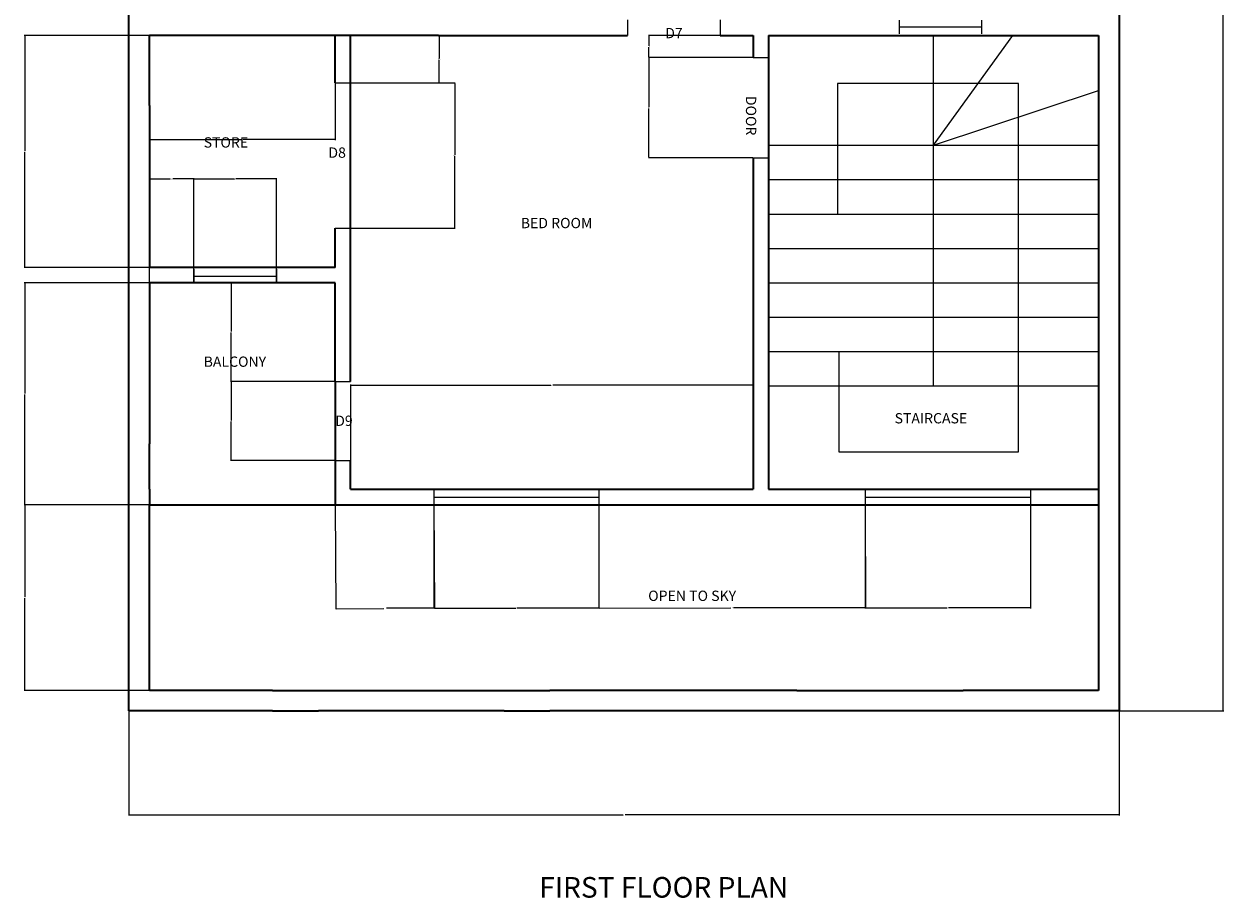
# Model space of a CAD drawing. Units: inches. Extents: x 301 to 1174, y -458 to 167.
# Tile 2 of 4: x 825 to 1174, y -458 to -203. Entities that reach past the tile are written whole.
import ezdxf

# ---------------------------------------------------------------- set-up
doc = ezdxf.new("R2010")
doc.units = ezdxf.units.IN
doc.header["$MEASUREMENT"] = 0
for name, color, linetype, lineweight in [('A-ANNO-DIMS', 2, 'Continuous', 18), ('A-ANNO-TEXT', 7, 'Continuous', 25), ('A-AREA-IDEN', 7, 'Continuous', 18), ('A-DOOR', 3, 'Continuous', 25), ('A-FLOR-STRS', 7, 'Continuous', 18), ('A-GLAZ', 4, 'Continuous', 18), ('A-WALL', 7, 'Continuous', 35)]:
    doc.layers.add(name, color=color, linetype=linetype, lineweight=lineweight)
doc.styles.get("Standard").update_dxf_attribs({"font": 'arial.ttf'})
doc.dimstyles.get("Standard").update_dxf_attribs({"dimtxt": 0.18, "dimasz": 0.18, "dimexe": 0.18, "dimexo": 0.0625, "dimgap": 0.09, "dimtad": 0, "dimtih": 1, "dimtoh": 1, "dimdec": 4, "dimzin": 0, "dimdsep": 46, "dimtxsty": 'Standard', "dimcen": 0.09, "dimadec": 0, "dimazin": 0, "dimtfac": 1, "dimtdec": 4, "dimtofl": 0, "dimtmove": 0, "dimatfit": 3, "dimfxl": 1, "dimtolj": 1, "dimtzin": 0, "dimarcsym": 0})

# ---------------------------------------------------------------- blocks, each defined once
blk = doc.blocks.new('*U2')
for p, q in [((0, 4), (0, 0)), ((24, 4), (24, 0)), ((0, 2), (24, 2))]:
    blk.add_line(p, q)
blk = doc.blocks.new('*U3')
for p, q in [((0, 4), (0, 0)), ((48, 4), (48, 0)), ((0, 2), (48, 2))]:
    blk.add_line(p, q)
blk = doc.blocks.new('STAIR-RES-WINDER')
for p, q in [((48, 19.16), (48, 121.12)), ((48, 89.16), (71.07, 121.12)), ((72.66, 107.09), (20.07, 107.09)), ((20.07, 107.09), (20.07, 69.16)), ((48, 89.16), (96, 105.1)), ((72.66, 0), (72.66, 107.09)), ((0, 89.16), (96, 89.16)), ((0, 79.16), (96, 79.16)), ((0, 69.16), (96, 69.16)), ((0, 59.16), (96, 59.16)), ((0, 49.16), (96, 49.16)), ((0, 39.16), (96, 39.16)), ((0, 29.16), (96, 29.16)), ((20.47, 29.16), (20.47, 0)), ((0, 19.16), (96, 19.16)), ((20.47, 0), (72.66, 0))]:
    blk.add_line(p, q)
blk = doc.blocks.new('*D38')
at = {"layer": 'A-ANNO-DIMS', "color": 0, "lineweight": -2, "transparency": 16777216}
for p, q in [((855.2, -403.26), (855.2, -433.63)), ((1143.2, -403.26), (1143.2, -433.63)), ((855.38, -433.45), (998.91, -433.45)), ((1143.02, -433.45), (999.49, -433.45))]:
    blk.add_line(p, q, dxfattribs=at)
at = {"layer": 'A-ANNO-DIMS', "color": 0, "transparency": 16777216}
for points in [[(855.38, -433.42), (855.38, -433.48), (855.2, -433.45)], [(1143.02, -433.42), (1143.02, -433.48), (1143.2, -433.45)]]:
    blk.add_solid(points, dxfattribs=at)
at = {"layer": 'Defpoints', "color": 0, "transparency": 16777216}
for p in [(855.2, -403.2), (1143.2, -403.2), (1143.2, -433.45)]:
    blk.add_point(p, dxfattribs=at)
at = {"layer": 'A-ANNO-DIMS', "color": 0, "transparency": 16777216, "insert": (999.2, -433.45), "char_height": 0.18, "attachment_point": 5}
blk.add_mtext('\\A1;288', dxfattribs=at)
blk = doc.blocks.new('*D39')
at = {"layer": 'A-ANNO-DIMS', "color": 0, "lineweight": -2, "transparency": 16777216}
for p, q in [((1143.26, 136.8), (1173.63, 136.8)), ((1173.45, 136.62), (1173.45, -133.02)), ((1173.45, -403.02), (1173.45, -133.38)), ((1143.26, -403.2), (1173.63, -403.2))]:
    blk.add_line(p, q, dxfattribs=at)
at = {"layer": 'A-ANNO-DIMS', "color": 0, "transparency": 16777216}
for points in [[(1173.42, 136.62), (1173.48, 136.62), (1173.45, 136.8)], [(1173.42, -403.02), (1173.48, -403.02), (1173.45, -403.2)]]:
    blk.add_solid(points, dxfattribs=at)
at = {"layer": 'Defpoints', "color": 0, "transparency": 16777216}
for p in [(1143.2, 136.8), (1173.45, 136.8), (1143.2, -403.2)]:
    blk.add_point(p, dxfattribs=at)
at = {"layer": 'A-ANNO-DIMS', "color": 0, "transparency": 16777216, "insert": (1173.45, -133.2), "char_height": 0.18, "attachment_point": 5}
blk.add_mtext('\\A1;540', dxfattribs=at)
blk = doc.blocks.new('*D53')
at = {"layer": 'A-ANNO-DIMS', "color": 0, "lineweight": -2, "transparency": 16777216}
for p, q in [((861.2, -206.76), (861.2, -237.13)), ((915.2, -206.76), (915.2, -237.13)), ((861.38, -236.95), (887.98, -236.95)), ((915.02, -236.95), (888.42, -236.95))]:
    blk.add_line(p, q, dxfattribs=at)
at = {"layer": 'A-ANNO-DIMS', "color": 0, "transparency": 16777216}
for points in [[(861.38, -236.92), (861.38, -236.98), (861.2, -236.95)], [(915.02, -236.92), (915.02, -236.98), (915.2, -236.95)]]:
    blk.add_solid(points, dxfattribs=at)
at = {"layer": 'Defpoints', "color": 0, "transparency": 16777216}
for p in [(861.2, -206.7), (915.2, -206.7), (861.2, -236.95)]:
    blk.add_point(p, dxfattribs=at)
at = {"layer": 'A-ANNO-DIMS', "color": 0, "transparency": 16777216, "insert": (888.2, -236.95), "char_height": 0.18, "attachment_point": 5}
blk.add_mtext('\\A1;54', dxfattribs=at)
blk = doc.blocks.new('*D54')
at = {"layer": 'A-ANNO-DIMS', "color": 0, "lineweight": -2, "transparency": 16777216}
for p, q in [((919.7, -338.64), (919.7, -308.27)), ((919.88, -308.45), (977.92, -308.45)), ((1036.52, -308.45), (978.48, -308.45)), ((1036.7, -338.64), (1036.7, -308.27))]:
    blk.add_line(p, q, dxfattribs=at)
at = {"layer": 'A-ANNO-DIMS', "color": 0, "transparency": 16777216}
for points in [[(919.88, -308.42), (919.88, -308.48), (919.7, -308.45)], [(1036.52, -308.42), (1036.52, -308.48), (1036.7, -308.45)]]:
    blk.add_solid(points, dxfattribs=at)
at = {"layer": 'Defpoints', "color": 0, "transparency": 16777216}
for p in [(1036.7, -308.45), (919.7, -338.7), (1036.7, -338.7)]:
    blk.add_point(p, dxfattribs=at)
at = {"layer": 'A-ANNO-DIMS', "color": 0, "transparency": 16777216, "insert": (978.2, -308.45), "char_height": 0.18, "attachment_point": 5}
blk.add_mtext('\\A1;117', dxfattribs=at)
blk = doc.blocks.new('*D63')
at = {"layer": 'A-ANNO-DIMS', "color": 0, "lineweight": -2, "transparency": 16777216}
for p, q in [((861.13, -206.7), (824.77, -206.7)), ((824.95, -206.88), (824.95, -240.27)), ((824.95, -274.02), (824.95, -240.63)), ((861.13, -274.2), (824.77, -274.2))]:
    blk.add_line(p, q, dxfattribs=at)
at = {"layer": 'A-ANNO-DIMS', "color": 0, "transparency": 16777216}
for points in [[(824.92, -206.88), (824.98, -206.88), (824.95, -206.7)], [(824.92, -274.02), (824.98, -274.02), (824.95, -274.2)]]:
    blk.add_solid(points, dxfattribs=at)
at = {"layer": 'Defpoints', "color": 0, "transparency": 16777216}
for p in [(824.95, -206.7), (861.2, -206.7), (861.2, -274.2)]:
    blk.add_point(p, dxfattribs=at)
at = {"layer": 'A-ANNO-DIMS', "color": 0, "transparency": 16777216, "insert": (824.95, -240.45), "char_height": 0.18, "attachment_point": 5}
blk.add_mtext('\\A1;67.5', dxfattribs=at)
blk = doc.blocks.new('*D64')
at = {"layer": 'A-ANNO-DIMS', "color": 0, "lineweight": -2, "transparency": 16777216}
for p, q in [((861.13, -278.7), (824.77, -278.7)), ((824.95, -278.88), (824.95, -310.77)), ((824.95, -343.02), (824.95, -311.13)), ((861.13, -343.2), (824.77, -343.2))]:
    blk.add_line(p, q, dxfattribs=at)
at = {"layer": 'A-ANNO-DIMS', "color": 0, "transparency": 16777216}
for points in [[(824.92, -278.88), (824.98, -278.88), (824.95, -278.7)], [(824.92, -343.02), (824.98, -343.02), (824.95, -343.2)]]:
    blk.add_solid(points, dxfattribs=at)
at = {"layer": 'Defpoints', "color": 0, "transparency": 16777216}
for p in [(824.95, -278.7), (861.2, -278.7), (861.2, -343.2)]:
    blk.add_point(p, dxfattribs=at)
at = {"layer": 'A-ANNO-DIMS', "color": 0, "transparency": 16777216, "insert": (824.95, -310.95), "char_height": 0.18, "attachment_point": 5}
blk.add_mtext('\\A1;64.5', dxfattribs=at)
blk = doc.blocks.new('*D65')
at = {"layer": 'A-ANNO-DIMS', "color": 0, "lineweight": -2, "transparency": 16777216}
for p, q in [((861.13, -343.2), (824.77, -343.2)), ((824.95, -343.38), (824.95, -370.02)), ((824.95, -397.02), (824.95, -370.38)), ((861.13, -397.2), (824.77, -397.2))]:
    blk.add_line(p, q, dxfattribs=at)
at = {"layer": 'A-ANNO-DIMS', "color": 0, "transparency": 16777216}
for points in [[(824.92, -343.38), (824.98, -343.38), (824.95, -343.2)], [(824.92, -397.02), (824.98, -397.02), (824.95, -397.2)]]:
    blk.add_solid(points, dxfattribs=at)
at = {"layer": 'Defpoints', "color": 0, "transparency": 16777216}
for p in [(824.95, -343.2), (861.2, -343.2), (861.2, -397.2)]:
    blk.add_point(p, dxfattribs=at)
at = {"layer": 'A-ANNO-DIMS', "color": 0, "transparency": 16777216, "insert": (824.95, -370.2), "char_height": 0.18, "attachment_point": 5}
blk.add_mtext('\\A1;54', dxfattribs=at)
blk = doc.blocks.new('*D91')
at = {"layer": 'A-ANNO-DIMS', "color": 0, "lineweight": -2, "transparency": 16777216}
for p, q in [((915.26, -206.7), (945.63, -206.7)), ((945.45, -206.88), (945.45, -213.41)), ((945.45, -220.3), (945.45, -213.77)), ((915.26, -220.48), (945.63, -220.48))]:
    blk.add_line(p, q, dxfattribs=at)
at = {"layer": 'A-ANNO-DIMS', "color": 0, "transparency": 16777216}
for points in [[(945.42, -206.88), (945.48, -206.88), (945.45, -206.7)], [(945.42, -220.3), (945.48, -220.3), (945.45, -220.48)]]:
    blk.add_solid(points, dxfattribs=at)
at = {"layer": 'Defpoints', "color": 0, "transparency": 16777216}
for p in [(915.2, -206.7), (915.2, -220.48), (945.45, -220.48)]:
    blk.add_point(p, dxfattribs=at)
at = {"layer": 'A-ANNO-DIMS', "color": 0, "transparency": 16777216, "insert": (945.45, -213.59), "char_height": 0.18, "attachment_point": 5}
blk.add_mtext('\\A1;13.784', dxfattribs=at)
blk = doc.blocks.new('*D92')
at = {"layer": 'A-ANNO-DIMS', "color": 0, "lineweight": -2, "transparency": 16777216}
for p, q in [((919.76, -220.48), (950.13, -220.48)), ((949.95, -220.66), (949.95, -241.43)), ((949.95, -262.56), (949.95, -241.79)), ((919.76, -262.74), (950.13, -262.74))]:
    blk.add_line(p, q, dxfattribs=at)
at = {"layer": 'A-ANNO-DIMS', "color": 0, "transparency": 16777216}
for points in [[(949.92, -220.66), (949.98, -220.66), (949.95, -220.48)], [(949.92, -262.56), (949.98, -262.56), (949.95, -262.74)]]:
    blk.add_solid(points, dxfattribs=at)
at = {"layer": 'Defpoints', "color": 0, "transparency": 16777216}
for p in [(919.7, -220.48), (919.7, -262.74), (949.95, -262.74)]:
    blk.add_point(p, dxfattribs=at)
at = {"layer": 'A-ANNO-DIMS', "color": 0, "transparency": 16777216, "insert": (949.95, -241.61), "char_height": 0.18, "attachment_point": 5}
blk.add_mtext('\\A1;42.256', dxfattribs=at)
blk = doc.blocks.new('*D93')
at = {"layer": 'A-ANNO-DIMS', "color": 0, "lineweight": -2, "transparency": 16777216}
for p, q in [((915.13, -307.34), (884.77, -307.34)), ((884.95, -307.52), (884.95, -318.68)), ((884.95, -330.21), (884.95, -319.05)), ((915.13, -330.39), (884.77, -330.39))]:
    blk.add_line(p, q, dxfattribs=at)
at = {"layer": 'A-ANNO-DIMS', "color": 0, "transparency": 16777216}
for points in [[(884.92, -307.52), (884.98, -307.52), (884.95, -307.34)], [(884.92, -330.21), (884.98, -330.21), (884.95, -330.39)]]:
    blk.add_solid(points, dxfattribs=at)
at = {"layer": 'Defpoints', "color": 0, "transparency": 16777216}
for p in [(884.95, -307.34), (915.2, -307.34), (915.2, -330.39)]:
    blk.add_point(p, dxfattribs=at)
at = {"layer": 'A-ANNO-DIMS', "color": 0, "transparency": 16777216, "insert": (884.95, -318.86), "char_height": 0.18, "attachment_point": 5}
blk.add_mtext('\\A1;23.055', dxfattribs=at)
blk = doc.blocks.new('*D94')
at = {"layer": 'A-ANNO-DIMS', "color": 0, "lineweight": -2, "transparency": 16777216}
for p, q in [((915.13, -278.7), (884.77, -278.7)), ((884.95, -278.88), (884.95, -292.84)), ((884.95, -307.16), (884.95, -293.2)), ((915.13, -307.34), (884.77, -307.34))]:
    blk.add_line(p, q, dxfattribs=at)
at = {"layer": 'A-ANNO-DIMS', "color": 0, "transparency": 16777216}
for points in [[(884.92, -278.88), (884.98, -278.88), (884.95, -278.7)], [(884.92, -307.16), (884.98, -307.16), (884.95, -307.34)]]:
    blk.add_solid(points, dxfattribs=at)
at = {"layer": 'Defpoints', "color": 0, "transparency": 16777216}
for p in [(884.95, -278.7), (915.2, -278.7), (915.2, -307.34)]:
    blk.add_point(p, dxfattribs=at)
at = {"layer": 'A-ANNO-DIMS', "color": 0, "transparency": 16777216, "insert": (884.95, -293.02), "char_height": 0.18, "attachment_point": 5}
blk.add_mtext('\\A1;28.637', dxfattribs=at)
blk = doc.blocks.new('*D95')
at = {"layer": 'A-ANNO-DIMS', "color": 0, "lineweight": -2, "transparency": 16777216}
for p, q in [((1036.63, -213.17), (1006.27, -213.17)), ((1006.45, -213.35), (1006.45, -227.56)), ((1006.45, -242.14), (1006.45, -227.93)), ((1036.63, -242.32), (1006.27, -242.32))]:
    blk.add_line(p, q, dxfattribs=at)
at = {"layer": 'A-ANNO-DIMS', "color": 0, "transparency": 16777216}
for points in [[(1006.42, -213.35), (1006.48, -213.35), (1006.45, -213.17)], [(1006.42, -242.14), (1006.48, -242.14), (1006.45, -242.32)]]:
    blk.add_solid(points, dxfattribs=at)
at = {"layer": 'Defpoints', "color": 0, "transparency": 16777216}
for p in [(1006.45, -213.17), (1036.7, -213.17), (1036.7, -242.32)]:
    blk.add_point(p, dxfattribs=at)
at = {"layer": 'A-ANNO-DIMS', "color": 0, "transparency": 16777216, "insert": (1006.45, -227.74), "char_height": 0.18, "attachment_point": 5}
blk.add_mtext('\\A1;29.16', dxfattribs=at)
blk = doc.blocks.new('*D96')
at = {"layer": 'A-ANNO-DIMS', "color": 0, "lineweight": -2, "transparency": 16777216}
for p, q in [((1036.63, -206.7), (1006.27, -206.7)), ((1006.45, -206.88), (1006.45, -209.75)), ((1006.45, -212.99), (1006.45, -210.11)), ((1036.63, -213.17), (1006.27, -213.17))]:
    blk.add_line(p, q, dxfattribs=at)
at = {"layer": 'A-ANNO-DIMS', "color": 0, "transparency": 16777216}
for points in [[(1006.42, -206.88), (1006.48, -206.88), (1006.45, -206.7)], [(1006.42, -212.99), (1006.48, -212.99), (1006.45, -213.17)]]:
    blk.add_solid(points, dxfattribs=at)
at = {"layer": 'Defpoints', "color": 0, "transparency": 16777216}
for p in [(1006.45, -206.7), (1036.7, -206.7), (1036.7, -213.17)]:
    blk.add_point(p, dxfattribs=at)
at = {"layer": 'A-ANNO-DIMS', "color": 0, "transparency": 16777216, "insert": (1006.45, -209.93), "char_height": 0.18, "attachment_point": 5}
blk.add_mtext('\\A1;6.467', dxfattribs=at)
blk = doc.blocks.new('*D97')
at = {"layer": 'A-ANNO-DIMS', "color": 0, "lineweight": -2, "transparency": 16777216}
for p, q in [((915.2, -343.26), (915.41, -373.63)), ((943.91, -343.06), (944.12, -373.43)), ((915.59, -373.45), (929.39, -373.35)), ((943.94, -373.25), (930.14, -373.34))]:
    blk.add_line(p, q, dxfattribs=at)
at = {"layer": 'A-ANNO-DIMS', "color": 0, "transparency": 16777216}
for points in [[(943.94, -373.22), (943.94, -373.28), (944.12, -373.25)], [(915.59, -373.42), (915.59, -373.48), (915.41, -373.45)]]:
    blk.add_solid(points, dxfattribs=at)
at = {"layer": 'Defpoints', "color": 0, "transparency": 16777216}
for p in [(915.2, -343.2), (943.9, -343), (915.41, -373.45)]:
    blk.add_point(p, dxfattribs=at)
at = {"layer": 'A-ANNO-DIMS', "color": 0, "transparency": 16777216, "insert": (929.76, -373.35), "char_height": 0.18, "attachment_point": 5}
blk.add_mtext('\\A1;28.71', dxfattribs=at)
blk = doc.blocks.new('*D98')
at = {"layer": 'A-ANNO-DIMS', "color": 0, "lineweight": -2, "transparency": 16777216}
for p, q in [((943.9, -343.06), (943.9, -373.43)), ((991.9, -343.06), (991.9, -373.43)), ((944.08, -373.25), (967.68, -373.25)), ((991.72, -373.25), (968.13, -373.25))]:
    blk.add_line(p, q, dxfattribs=at)
at = {"layer": 'A-ANNO-DIMS', "color": 0, "transparency": 16777216}
for points in [[(944.08, -373.22), (944.08, -373.28), (943.9, -373.25)], [(991.72, -373.22), (991.72, -373.28), (991.9, -373.25)]]:
    blk.add_solid(points, dxfattribs=at)
at = {"layer": 'Defpoints', "color": 0, "transparency": 16777216}
for p in [(943.9, -343), (991.9, -343), (943.9, -373.25)]:
    blk.add_point(p, dxfattribs=at)
at = {"layer": 'A-ANNO-DIMS', "color": 0, "transparency": 16777216, "insert": (967.9, -373.25), "char_height": 0.18, "attachment_point": 5}
blk.add_mtext('\\A1;48', dxfattribs=at)
blk = doc.blocks.new('*D99')
at = {"layer": 'A-ANNO-DIMS', "color": 0, "lineweight": -2, "transparency": 16777216}
for p, q in [((991.9, -343.06), (991.91, -373.43)), ((1069.35, -343.05), (1069.36, -373.42)), ((992.09, -373.25), (1030.24, -373.24)), ((1069.18, -373.24), (1031.03, -373.24))]:
    blk.add_line(p, q, dxfattribs=at)
at = {"layer": 'A-ANNO-DIMS', "color": 0, "transparency": 16777216}
for points in [[(992.09, -373.22), (992.09, -373.28), (991.91, -373.25)], [(1069.18, -373.21), (1069.18, -373.27), (1069.36, -373.24)]]:
    blk.add_solid(points, dxfattribs=at)
at = {"layer": 'Defpoints', "color": 0, "transparency": 16777216}
for p in [(991.9, -343), (1069.35, -342.99), (991.91, -373.25)]:
    blk.add_point(p, dxfattribs=at)
at = {"layer": 'A-ANNO-DIMS', "color": 0, "transparency": 16777216, "insert": (1030.63, -373.24), "char_height": 0.18, "attachment_point": 5}
blk.add_mtext('\\A1;77.45', dxfattribs=at)
blk = doc.blocks.new('*D100')
at = {"layer": 'A-ANNO-DIMS', "color": 0, "lineweight": -2, "transparency": 16777216}
for p, q in [((1069.35, -343.05), (1069.35, -373.42)), ((1117.35, -343.05), (1117.35, -373.42)), ((1069.53, -373.24), (1093.13, -373.24)), ((1117.17, -373.24), (1093.58, -373.24))]:
    blk.add_line(p, q, dxfattribs=at)
at = {"layer": 'A-ANNO-DIMS', "color": 0, "transparency": 16777216}
for points in [[(1069.53, -373.21), (1069.53, -373.27), (1069.35, -373.24)], [(1117.17, -373.21), (1117.17, -373.27), (1117.35, -373.24)]]:
    blk.add_solid(points, dxfattribs=at)
at = {"layer": 'Defpoints', "color": 0, "transparency": 16777216}
for p in [(1069.35, -342.99), (1117.35, -342.99), (1069.35, -373.24)]:
    blk.add_point(p, dxfattribs=at)
at = {"layer": 'A-ANNO-DIMS', "color": 0, "transparency": 16777216, "insert": (1093.35, -373.24), "char_height": 0.18, "attachment_point": 5}
blk.add_mtext('\\A1;48', dxfattribs=at)
blk = doc.blocks.new('*D101')
at = {"layer": 'A-ANNO-DIMS', "color": 0, "lineweight": -2, "transparency": 16777216}
for p, q in [((861.2, -278.64), (861.18, -248.27)), ((861.36, -248.45), (867.26, -248.45)), ((873.92, -248.44), (868.03, -248.45)), ((874.12, -278.63), (874.1, -248.26))]:
    blk.add_line(p, q, dxfattribs=at)
at = {"layer": 'A-ANNO-DIMS', "color": 0, "transparency": 16777216}
for points in [[(861.36, -248.42), (861.36, -248.48), (861.18, -248.45)], [(873.92, -248.41), (873.92, -248.47), (874.1, -248.44)]]:
    blk.add_solid(points, dxfattribs=at)
at = {"layer": 'Defpoints', "color": 0, "transparency": 16777216}
for p in [(874.1, -248.44), (861.2, -278.7), (874.12, -278.69)]:
    blk.add_point(p, dxfattribs=at)
at = {"layer": 'A-ANNO-DIMS', "color": 0, "transparency": 16777216, "insert": (867.64, -248.45), "char_height": 0.18, "attachment_point": 5}
blk.add_mtext('\\A1;12.92', dxfattribs=at)
blk = doc.blocks.new('*D102')
at = {"layer": 'A-ANNO-DIMS', "color": 0, "lineweight": -2, "transparency": 16777216}
for p, q in [((874.12, -278.63), (874.12, -248.26)), ((874.3, -248.44), (885.9, -248.44)), ((897.94, -248.44), (886.34, -248.44)), ((898.12, -278.63), (898.12, -248.26))]:
    blk.add_line(p, q, dxfattribs=at)
at = {"layer": 'A-ANNO-DIMS', "color": 0, "transparency": 16777216}
for points in [[(874.3, -248.41), (874.3, -248.47), (874.12, -248.44)], [(897.94, -248.41), (897.94, -248.47), (898.12, -248.44)]]:
    blk.add_solid(points, dxfattribs=at)
at = {"layer": 'Defpoints', "color": 0, "transparency": 16777216}
for p in [(898.12, -248.44), (874.12, -278.69), (898.12, -278.69)]:
    blk.add_point(p, dxfattribs=at)
at = {"layer": 'A-ANNO-DIMS', "color": 0, "transparency": 16777216, "insert": (886.12, -248.44), "char_height": 0.18, "attachment_point": 5}
blk.add_mtext('\\A1;24', dxfattribs=at)

msp = doc.modelspace()

# ---------------------------------------------------------------- linework, layer by layer
at = {"layer": 'A-DOOR'}
for p, q in [((1000.233, -202.1987), (1000.233, -206.6987)), ((1027.1125, -202.1987), (1027.1125, -206.6987)), ((1036.6974, -213.1652), (1041.1974, -213.1652)), ((915.1974, -220.4828), (919.6974, -220.4828)), ((1036.6974, -242.3233), (1041.1974, -242.3233)), ((915.1974, -262.7385), (919.6974, -262.7385)), ((915.1974, -307.3357), (919.6974, -307.3357)), ((915.1974, -330.3907), (919.6974, -330.3907))]:
    msp.add_line(p, q, dxfattribs=at)
at = {"layer": 'A-WALL'}
for p, q in [((855.1974, -403.1987), (855.1974, 136.8013)), ((1143.1974, 136.8013), (1143.1974, -403.1987)), ((861.1974, -227.0735), (861.1974, -206.6987)), ((945.1974, -206.6987), (861.1974, -206.6987)), ((915.1974, -220.4828), (915.1974, -206.6987)), ((919.6974, -307.3357), (919.6974, -206.6987)), ((945.1974, -206.6987), (1000.233, -206.6987)), ((1027.1125, -206.6987), (1036.6974, -206.6987)), ((1036.6974, -206.6987), (1036.6974, -213.1652)), ((1041.1974, -206.6987), (1137.1974, -206.6987)), ((1041.1974, -206.6987), (1041.1974, -338.6987)), ((1137.1974, -206.6987), (1137.1974, -397.1987)), ((861.1974, -227.0735), (861.1974, -274.1987)), ((1036.6974, -242.3233), (1036.6974, -338.6987)), ((915.1974, -274.1987), (915.1974, -262.7385)), ((915.1974, -274.1987), (861.1974, -274.1987)), ((915.1974, -278.6987), (861.1974, -278.6987)), ((861.1974, -278.6987), (861.1974, -325.5087)), ((915.1974, -307.3357), (915.1974, -278.6987)), ((915.1974, -307.3357), (915.1974, -343.1987)), ((861.1974, -338.6987), (861.1974, -325.5087)), ((919.6974, -338.6987), (919.6974, -330.3907)), ((861.1974, -338.6987), (861.1974, -343.1987)), ((919.6974, -338.6987), (1036.6974, -338.6987)), ((1041.1974, -338.6987), (1137.1974, -338.6987)), ((861.1974, -397.1987), (861.1974, -343.1987)), ((861.1974, -343.1987), (1137.1974, -343.1987)), ((896.9826, -397.1987), (861.1974, -397.1987)), ((896.9826, -397.1987), (977.6563, -397.1987)), ((1049.3903, -397.1987), (977.6563, -397.1987)), ((1049.3903, -397.1987), (1097.8241, -397.1987)), ((1137.1974, -397.1987), (1097.8241, -397.1987)), ((896.9826, -403.1987), (855.1974, -403.1987)), ((896.9826, -403.1987), (910.3007, -403.1987)), ((964.3381, -403.1987), (910.3007, -403.1987)), ((964.3381, -403.1987), (977.6563, -403.1987)), ((1143.1974, -403.1987), (977.6563, -403.1987))]:
    msp.add_line(p, q, dxfattribs=at)

# ---------------------------------------------------------------- block references
at = {"layer": 'A-FLOR-STRS'}
msp.add_blockref('STAIR-RES-WINDER', (1041.1974, -327.8143), dxfattribs=at)
at = {"layer": 'A-GLAZ'}
for name, p in [('*U2', (1079.1778, -206.2439)), ('*U2', (874.1169, -278.6923)), ('*U3', (943.9048, -342.9958)), ('*U3', (1069.3525, -342.9853))]:
    msp.add_blockref(name, p, dxfattribs=at)

# ---------------------------------------------------------------- texts
at = {"layer": 'A-ANNO-TEXT', "attachment_point": 1}
for s, width, insert, char_height in [('D7', 13.351331, (1011.16, -204.5331), 3), ('D8', 13.351331, (913.2221, -239.2924), 3), ('D9', 13.351331, (915.1974, -317.2945), 3), ('FIRST FLOOR PLAN', 138.96688, (974.5321, -451.4928), 6)]:
    msp.add_mtext_dynamic_manual_height_columns(s, width=width, gutter_width=1, heights=[0], dxfattribs=dict(at, insert=insert, char_height=char_height))
at = {"layer": 'A-ANNO-TEXT', "insert": (1037.6289, -224.3005), "char_height": 3, "attachment_point": 1, "rotation": 270}
msp.add_mtext_dynamic_manual_height_columns('DOOR', width=13.351331, gutter_width=1, heights=[0], dxfattribs=at)
at = {"layer": 'A-AREA-IDEN', "char_height": 0.2, "attachment_point": 1}
for s, insert in [('{\\H15x;STORE}', (876.9433, -236.3361)), ('{\\H15x;BED ROOM}', (969.1676, -259.7851)), ('{\\H15x;BALCONY}', (876.9433, -300.1009)), ('{\\H15x;STAIRCASE}', (1077.8604, -316.5563)), ('{\\H15x;OPEN TO SKY}', (1006.2156, -368.2025))]:
    msp.add_mtext_dynamic_manual_height_columns(s, width=70.987625, gutter_width=1, heights=[0], dxfattribs=dict(at, insert=insert))

# ---------------------------------------------------------------- dimensions: what is measured, and where the dimension line sits
at = {"layer": 'A-ANNO-DIMS'}
for base, p1, p2, angle, override, picture, middle in [((1173.4474, 136.8013), (1143.1974, -403.1987), (1143.1974, 136.8013), 90, {"dimdec": 0, "dimlfac": 1, "dimrnd": 0, "dimzin": 0, "dimdsep": 46, "dimlunit": 2}, '*D39', (1173.4474, -133.1987)), ((824.9474, -206.6987), (861.1974, -274.1987), (861.1974, -206.6987), 90, {"dimdec": 1, "dimlfac": 1, "dimrnd": 0, "dimzin": 0, "dimdsep": 46, "dimlunit": 2}, '*D63', (824.9474, -240.4487)), ((861.1974, -236.9487), (915.1974, -206.6987), (861.1974, -206.6987), 180, {"dimdec": 0, "dimlfac": 1, "dimrnd": 0, "dimzin": 0, "dimdsep": 46, "dimlunit": 2}, '*D53', (888.1974, -236.9487)), ((945.4474, -220.4828), (915.1974, -206.6987), (915.1974, -220.4828), 270, {"dimdec": 3, "dimlfac": 1, "dimrnd": 0, "dimzin": 0, "dimdsep": 46, "dimlunit": 2}, '*D91', (945.4474, -213.5908)), ((1006.44744, -206.69869), (1036.69744, -213.16525), (1036.69744, -206.69869), 90, {"dimdec": 3, "dimlfac": 1, "dimrnd": 0, "dimzin": 0, "dimdsep": 46, "dimlunit": 2}, '*D96', (1006.44744, -209.93197)), ((1006.4474, -213.1652), (1036.6974, -242.3233), (1036.6974, -213.1652), 90, {"dimdec": 2, "dimlfac": 1, "dimrnd": 0, "dimzin": 0, "dimdsep": 46, "dimlunit": 2}, '*D95', (1006.4474, -227.7443)), ((949.9474, -262.7385), (919.6974, -220.4828), (919.6974, -262.7385), 270, {"dimdec": 3, "dimlfac": 1, "dimrnd": 0, "dimzin": 0, "dimdsep": 46, "dimlunit": 2}, '*D92', (949.9474, -241.6107)), ((874.102, -248.4423), (861.1974, -278.6987), (874.1169, -278.6923), 0.028184, {"dimdec": 2, "dimlfac": 1, "dimrnd": 0, "dimzin": 0, "dimdsep": 46, "dimlunit": 2}, '*D101', (867.6423, -248.4455)), ((824.9474, -278.6987), (861.1974, -343.1987), (861.1974, -278.6987), 90, {"dimdec": 1, "dimlfac": 1, "dimrnd": 0, "dimzin": 0, "dimdsep": 46, "dimlunit": 2}, '*D64', (824.9474, -310.9487)), ((884.9474, -278.6987), (915.1974, -307.3357), (915.1974, -278.6987), 90, {"dimdec": 3, "dimlfac": 1, "dimrnd": 0, "dimzin": 0, "dimdsep": 46, "dimlunit": 2}, '*D94', (884.9474, -293.0172)), ((884.9474, -307.3357), (915.1974, -330.3907), (915.1974, -307.3357), 90, {"dimdec": 3, "dimlfac": 1, "dimrnd": 0, "dimzin": 0, "dimdsep": 46, "dimlunit": 2}, '*D93', (884.9474, -318.8632)), ((824.9474, -343.1987), (861.1974, -397.1987), (861.1974, -343.1987), 90, {"dimdec": 0, "dimlfac": 1, "dimrnd": 0, "dimzin": 0, "dimdsep": 46, "dimlunit": 2}, '*D65', (824.9474, -370.1987)), ((915.4113, -373.4479), (943.9048, -342.9958), (915.1974, -343.1987), 180.404987, {"dimdec": 2, "dimlfac": 1, "dimrnd": 0, "dimzin": 0, "dimdsep": 46, "dimlunit": 2}, '*D97', (929.7649, -373.3465)), ((943.9048, -373.2458), (991.9048, -342.9958), (943.9048, -342.9958), 180, {"dimdec": 0, "dimlfac": 1, "dimrnd": 0, "dimzin": 0, "dimdsep": 46, "dimlunit": 2}, '*D98', (967.9048, -373.2458)), ((991.9089, -373.2458), (1069.3525, -342.9853), (991.9048, -342.9958), 180.007769, {"dimdec": 2, "dimlfac": 1, "dimrnd": 0, "dimzin": 0, "dimdsep": 46, "dimlunit": 2}, '*D99', (1030.6328, -373.2405)), ((1069.3525, -373.2353), (1117.3525, -342.9853), (1069.3525, -342.9853), 180, {"dimdec": 0, "dimlfac": 1, "dimrnd": 0, "dimzin": 0, "dimdsep": 46, "dimlunit": 2}, '*D100', (1093.3525, -373.2353))]:
    dim = msp.add_linear_dim(base=base, p1=p1, p2=p2, angle=angle, dimstyle='Standard', override=override, dxfattribs=at)
    dim.commit()
    dim.dimension.update_dxf_attribs({"geometry": picture, "text_midpoint": middle})
for base, p1, p2, picture, middle in [((898.1169, -248.4423), (874.1169, -278.6923), (898.1169, -278.6923), '*D102', (886.1169, -248.4423)), ((1036.6974, -308.4487), (919.6974, -338.6987), (1036.6974, -338.6987), '*D54', (978.1974, -308.4487)), ((1143.1974, -433.4487), (855.1974, -403.1987), (1143.1974, -403.1987), '*D38', (999.1974, -433.4487))]:
    dim = msp.add_linear_dim(base=base, p1=p1, p2=p2, dimstyle='Standard', override={"dimdec": 0, "dimlfac": 1, "dimrnd": 0, "dimzin": 0, "dimdsep": 46, "dimlunit": 2}, dxfattribs=at)
    dim.commit()
    dim.dimension.update_dxf_attribs({"geometry": picture, "text_midpoint": middle})

doc.saveas('drawing.dxf')
